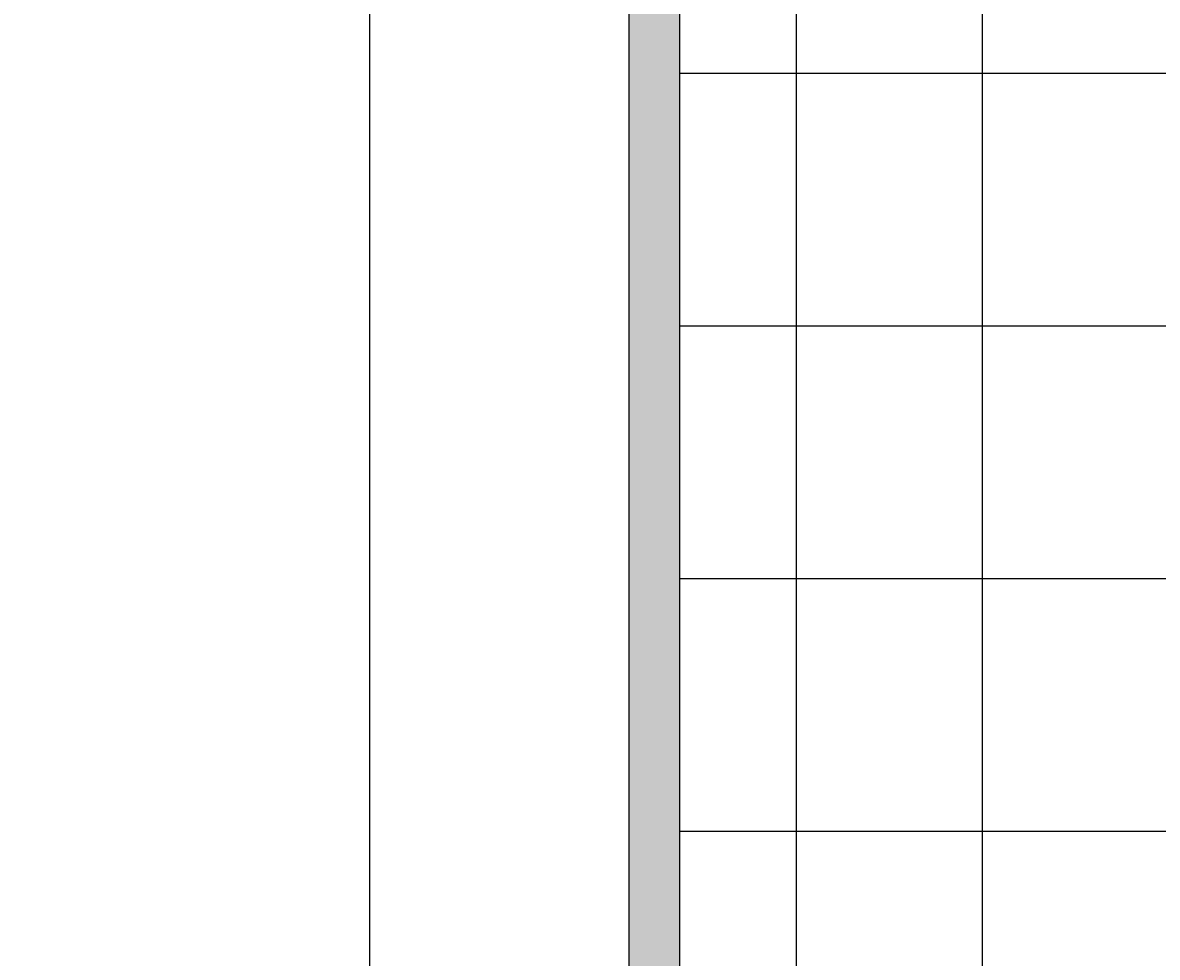
# Model space of a CAD drawing. Units: inches. Extents: x 2231 to 2461, y 2045 to 2455.
# Tile 59 of 95: x 2371 to 2416, y 2222 to 2259. Entities that reach past the tile are written whole.
import ezdxf

# ---------------------------------------------------------------- set-up
doc = ezdxf.new("R2010")
doc.units = ezdxf.units.IN
doc.layers.add('A-ANNO-DIMS', color=2, linetype='Continuous', lineweight=18)
doc.layers.add('A-FLOR-STRS', color=7, linetype='Continuous', lineweight=25)
doc.layers.add('A-WALL-PATT', color=18, linetype='Continuous', lineweight=13, true_color=0x000000)
doc.styles.get("Standard").update_dxf_attribs({"font": 'arial.ttf'})
doc.dimstyles.get("Standard").update_dxf_attribs({"dimtxt": 0.18, "dimasz": 0.18, "dimexe": 0.18, "dimexo": 0.0625, "dimgap": 0.09, "dimtad": 0, "dimtih": 1, "dimtoh": 1, "dimdec": 4, "dimzin": 0, "dimdsep": 46, "dimtxsty": 'Standard', "dimcen": 0.09, "dimadec": 0, "dimazin": 0, "dimtfac": 1, "dimtdec": 4, "dimtofl": 0, "dimtmove": 0, "dimatfit": 3, "dimfxl": 1, "dimtolj": 1, "dimtzin": 0, "dimarcsym": 0})

# ---------------------------------------------------------------- blocks, each defined once
blk = doc.blocks.new('*D59')
at = {"layer": 'A-ANNO-DIMS', "color": 0, "lineweight": -2, "transparency": 16777216}
for p, q in [((2408.794, 2182.895), (2408.794, 2454.645)), ((2408.974, 2454.465), (2420.573, 2454.465)), ((2432.614, 2454.465), (2421.014, 2454.465)), ((2432.794, 2182.895), (2432.794, 2454.645))]:
    blk.add_line(p, q, dxfattribs=at)
at = {"layer": 'A-ANNO-DIMS', "color": 0, "transparency": 16777216}
for points in [[(2408.974, 2454.495), (2408.974, 2454.435), (2408.794, 2454.465)], [(2432.614, 2454.495), (2432.614, 2454.435), (2432.794, 2454.465)]]:
    blk.add_solid(points, dxfattribs=at)
at = {"layer": 'Defpoints', "color": 0, "transparency": 16777216}
for p in [(2432.794, 2454.465), (2408.794, 2182.833), (2432.794, 2182.833)]:
    blk.add_point(p, dxfattribs=at)
at = {"layer": 'A-ANNO-DIMS', "color": 0, "transparency": 16777216, "insert": (2420.794, 2454.465), "char_height": 0.18, "attachment_point": 5}
blk.add_mtext('\\A1;24', dxfattribs=at)
blk = doc.blocks.new('*D66')
at = {"layer": 'A-ANNO-DIMS', "color": 0, "lineweight": -2, "transparency": 16777216}
for p, q in [((2348.189, 2096.895), (2348.189, 2454.645)), ((2348.369, 2454.465), (2378.167, 2454.465)), ((2408.614, 2454.465), (2378.815, 2454.465)), ((2408.794, 2096.895), (2408.794, 2454.645))]:
    blk.add_line(p, q, dxfattribs=at)
at = {"layer": 'A-ANNO-DIMS', "color": 0, "transparency": 16777216}
for points in [[(2348.369, 2454.495), (2348.369, 2454.435), (2348.189, 2454.465)], [(2408.614, 2454.495), (2408.614, 2454.435), (2408.794, 2454.465)]]:
    blk.add_solid(points, dxfattribs=at)
at = {"layer": 'Defpoints', "color": 0, "transparency": 16777216}
for p in [(2408.794, 2454.465), (2348.189, 2096.833), (2408.794, 2096.833)]:
    blk.add_point(p, dxfattribs=at)
at = {"layer": 'A-ANNO-DIMS', "color": 0, "transparency": 16777216, "insert": (2378.491, 2454.465), "char_height": 0.18, "attachment_point": 5}
blk.add_mtext('\\A1;60.6', dxfattribs=at)
blk = doc.blocks.new('*D71')
at = {"layer": 'A-ANNO-DIMS', "color": 0, "lineweight": -2, "transparency": 16777216}
for p, q in [((2401.422, 2092.979), (2401.422, 2454.645)), ((2401.602, 2454.465), (2404.732, 2454.465)), ((2408.614, 2454.465), (2405.483, 2454.465)), ((2408.794, 2096.895), (2408.794, 2454.645))]:
    blk.add_line(p, q, dxfattribs=at)
at = {"layer": 'A-ANNO-DIMS', "color": 0, "transparency": 16777216}
for points in [[(2401.602, 2454.495), (2401.602, 2454.435), (2401.422, 2454.465)], [(2408.614, 2454.495), (2408.614, 2454.435), (2408.794, 2454.465)]]:
    blk.add_solid(points, dxfattribs=at)
at = {"layer": 'Defpoints', "color": 0, "transparency": 16777216}
for p in [(2408.794, 2454.465), (2408.794, 2096.833), (2401.422, 2092.917)]:
    blk.add_point(p, dxfattribs=at)
at = {"layer": 'A-ANNO-DIMS', "color": 0, "transparency": 16777216, "insert": (2405.108, 2454.465), "char_height": 0.18, "attachment_point": 5}
blk.add_mtext('\\A1;7.371', dxfattribs=at)
blk = doc.blocks.new('*D72')
at = {"layer": 'A-ANNO-DIMS', "color": 0, "lineweight": -2, "transparency": 16777216}
for p, q in [((2384.543, 2145.12), (2384.543, 2454.645)), ((2384.723, 2454.465), (2396.272, 2454.465)), ((2408.614, 2454.465), (2397.064, 2454.465)), ((2408.794, 2150.677), (2408.794, 2454.645))]:
    blk.add_line(p, q, dxfattribs=at)
at = {"layer": 'A-ANNO-DIMS', "color": 0, "transparency": 16777216}
for points in [[(2384.723, 2454.495), (2384.723, 2454.435), (2384.543, 2454.465)], [(2408.614, 2454.495), (2408.614, 2454.435), (2408.794, 2454.465)]]:
    blk.add_solid(points, dxfattribs=at)
at = {"layer": 'Defpoints', "color": 0, "transparency": 16777216}
for p in [(2408.794, 2454.465), (2408.794, 2150.615), (2384.543, 2145.058)]:
    blk.add_point(p, dxfattribs=at)
at = {"layer": 'A-ANNO-DIMS', "color": 0, "transparency": 16777216, "insert": (2396.668, 2454.465), "char_height": 0.18, "attachment_point": 5}
blk.add_mtext('\\A1;24.25', dxfattribs=at)

msp = doc.modelspace()

# ---------------------------------------------------------------- hatches: boundary and pattern name
at = {"layer": 'A-WALL-PATT'}
h = msp.add_hatch(color=256, dxfattribs=at)
h.dxf.hatch_style = 1
h.paths.add_polyline_path([(2441.7935, 2269.1535), (2432.7935, 2269.1535), (2432.7935, 2186.8328), (2396.7935, 2186.8328), (2396.7935, 2286.8328), (2394.7935, 2286.8328), (2394.7935, 2186.8328), (2334.7935, 2186.8328), (2334.7935, 2182.8328), (2432.7935, 2182.8328), (2432.7935, 2072.8328), (2416.6639, 2072.8328), (2416.6639, 2063.8328), (2441.7935, 2063.8328)])
h.paths.add_polyline_path([(2368.6639, 2072.8328), (2367.04, 2072.8328), (2330.7942, 2072.8328), (2330.7397, 2063.8328), (2368.6639, 2063.8328)])
h.paths.add_polyline_path([(2300.7392, 2068.3328), (2300.7392, 2072.8328), (2298.7935, 2072.8328), (2294.7935, 2072.8328), (2258.7935, 2072.8328), (2258.7935, 2120.8328), (2294.7935, 2120.8328), (2298.7935, 2120.8328), (2298.7935, 2128.8328), (2294.7935, 2128.8328), (2294.7935, 2124.8328), (2258.7935, 2124.8328), (2258.7935, 2182.8328), (2294.7935, 2182.8328), (2294.7935, 2174.8328), (2298.7935, 2174.8328), (2298.7935, 2182.8328), (2304.7935, 2182.8328), (2304.7935, 2186.8328), (2258.7935, 2186.8328), (2258.7935, 2221.999), (2249.7935, 2221.999), (2249.7935, 2063.8328), (2300.7392, 2063.8328)])
h.paths.add_polyline_path([(2391.9338, 2435.8328), (2333.82, 2435.8328), (2333.82, 2426.8328), (2368.7935, 2426.8328), (2368.7935, 2374.9508), (2368.7935, 2370.8328), (2372.3935, 2370.8328), (2372.7935, 2370.8328), (2372.7935, 2426.8328), (2391.9338, 2426.8328)])
h.paths.add_polyline_path([(2441.7935, 2435.8328), (2415.9338, 2435.8328), (2415.9338, 2426.8328), (2432.7935, 2426.8328), (2432.7935, 2334.8328), (2372.7935, 2334.8328), (2372.7935, 2346.8328), (2368.7935, 2346.8328), (2368.7935, 2306.8328), (2360.7935, 2306.8328), (2360.7935, 2302.8328), (2368.7935, 2302.8328), (2372.7935, 2302.8328), (2372.7935, 2330.8328), (2432.7935, 2330.8328), (2432.7935, 2317.1535), (2441.7935, 2317.1535)])
h.paths.add_polyline_path([(2285.82, 2435.8328), (2249.7935, 2435.8328), (2249.7935, 2269.999), (2258.7935, 2269.999), (2258.7935, 2302.8328), (2318.8168, 2302.8328), (2330.7935, 2302.8328), (2330.7935, 2306.8328), (2258.7935, 2306.8328), (2258.7935, 2426.8328), (2285.82, 2426.8328)])

# ---------------------------------------------------------------- linework, layer by layer
at = {"layer": 'A-FLOR-STRS'}
for p, q in [((2394.7935, 2286.8328), (2394.7935, 2186.8328)), ((2396.7935, 2286.8328), (2396.7935, 2186.8328)), ((2396.7935, 2256.8328), (2432.7935, 2256.8328)), ((2396.7935, 2246.8328), (2432.7935, 2246.8328)), ((2396.7935, 2236.8328), (2432.7935, 2236.8328)), ((2396.7935, 2226.8328), (2432.7935, 2226.8328))]:
    msp.add_line(p, q, dxfattribs=at)

# ---------------------------------------------------------------- dimensions: what is measured, and where the dimension line sits
at = {"layer": 'A-ANNO-DIMS'}
for base, p1, p2, override, picture, middle in [((2408.7935, 2454.4653), (2348.1888, 2096.8328), (2408.7935, 2096.8328), {"dimdec": 1, "dimlfac": 1, "dimrnd": 0, "dimzin": 0, "dimdsep": 46, "dimlunit": 2}, '*D66', (2378.4912, 2454.4653)), ((2408.7935, 2454.4653), (2384.5428, 2145.0576), (2408.7935, 2150.6145), {"dimdec": 2, "dimlfac": 1, "dimrnd": 0, "dimzin": 0, "dimdsep": 46, "dimlunit": 2}, '*D72', (2396.6682, 2454.4653)), ((2408.7935, 2454.4653), (2401.4221, 2092.9167), (2408.7935, 2096.8328), {"dimdec": 3, "dimlfac": 1, "dimrnd": 0, "dimzin": 0, "dimdsep": 46, "dimlunit": 2}, '*D71', (2405.1078, 2454.4653)), ((2432.7935, 2454.4653), (2408.7935, 2182.8328), (2432.7935, 2182.8328), {"dimdec": 0, "dimlfac": 1, "dimrnd": 0, "dimzin": 0, "dimdsep": 46, "dimlunit": 2}, '*D59', (2420.7935, 2454.4653))]:
    dim = msp.add_linear_dim(base=base, p1=p1, p2=p2, dimstyle='Standard', override=override, dxfattribs=at)
    dim.commit()
    dim.dimension.update_dxf_attribs({"geometry": picture, "text_midpoint": middle})

doc.saveas('drawing.dxf')
